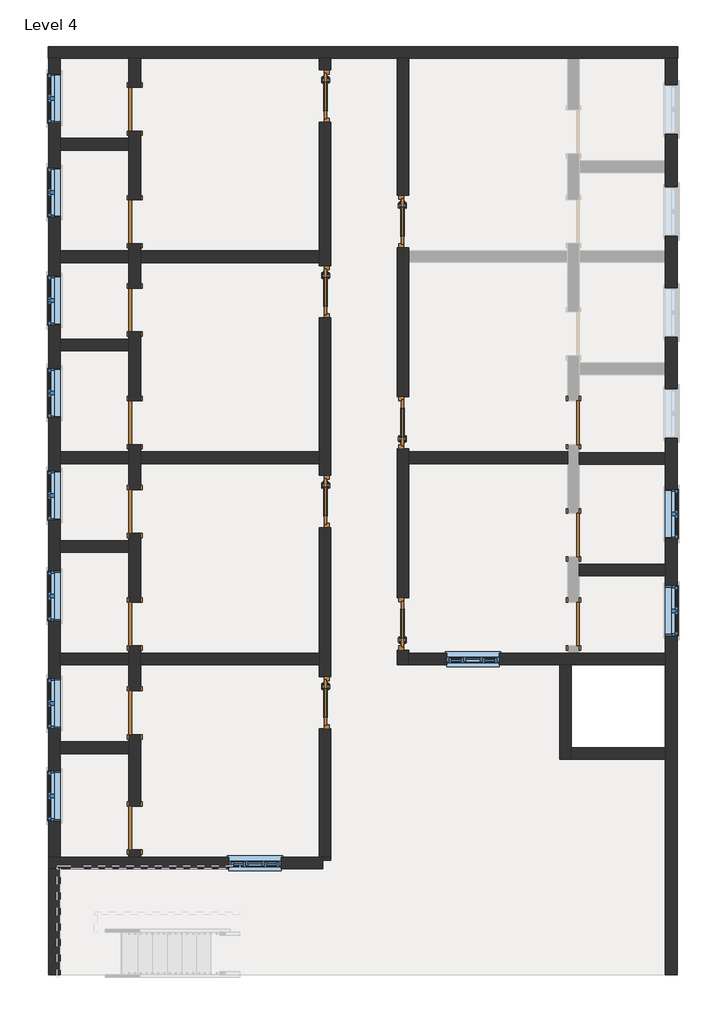
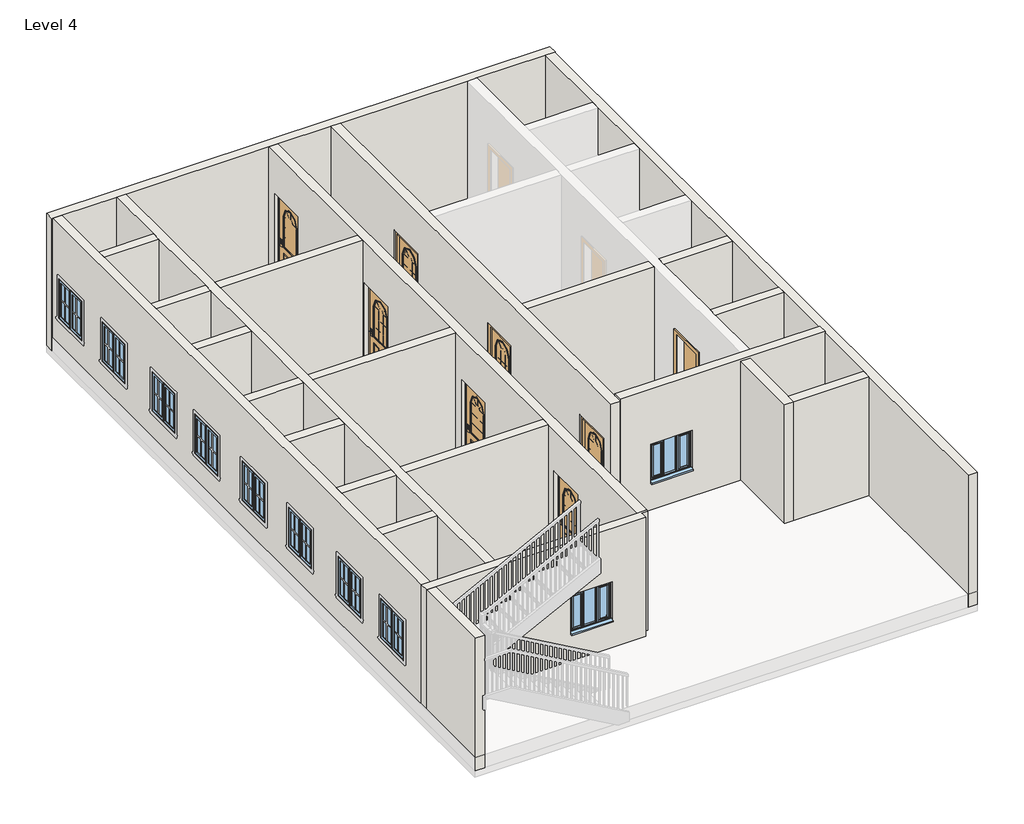
# One storey, part 1 of 4: 24 walls, 18 doors, 12 windows.
"""IFC4 building model written with IfcOpenShell, lengths in millimetres."""

from ifc_helpers import new_model, si_unit, frame, origin, place, context, project, spatial, polyline, outline, extrude, faceted_brep, transform, mapped, element, save
from components import doors_extsgl_w_glazing_bars_arched_910x2110mm_1ab485ba, doors_extsgl_w_glazing_bars_arched_910x2110mm_97dcda8a, door_fadea3f2, door_53b1b562, window_c29befe5, windows_tpl_plain_910x910mm_84e79c20

model = new_model("IFC4")

# Units and contexts
model_context = context("Model", 3, world=origin())
ifc_project = project(units=[si_unit("LENGTHUNIT", "METRE", prefix="MILLI")], contexts=[model_context])

# Site, building, storey
site = spatial("IfcSite", under=ifc_project)
building = spatial("IfcBuilding", under=site)
storey = spatial("IfcBuildingStorey", under=building, Name="Level 4", Elevation=9144.0)

# Doors
placement = place(None, origin())
doors_extsgl_w_glazing_bars_arched_910x2110mm_shape = doors_extsgl_w_glazing_bars_arched_910x2110mm_1ab485ba(model_context)
element("IfcDoor", 1, ObjectType="Doors_ExtSgl_w-Glazing_Bars_Arched : 910x2110mm", at=placement, inside=storey, context=model_context, shape_type="MappedRepresentation", body=[
    mapped(doors_extsgl_w_glazing_bars_arched_910x2110mm_shape, transform((-1635.1108866, 7135.2399728, 9144.0), x_axis=(0.0, -1.0, 0.0), y_axis=(1.0, 0.0, 0.0), z_axis=(0.0, 0.0, 1.0))),
])
element("IfcDoor", 2, ObjectType="Doors_ExtSgl_w-Glazing_Bars_Arched : 910x2110mm", at=placement, inside=storey, context=model_context, shape_type="MappedRepresentation", body=[
    mapped(doors_extsgl_w_glazing_bars_arched_910x2110mm_shape, transform((-1635.1108866, 3727.1935874, 9144.0), x_axis=(0.0, -1.0, 0.0), y_axis=(1.0, 0.0, 0.0), z_axis=(0.0, 0.0, 1.0))),
])
element("IfcDoor", 3, ObjectType="Doors_ExtSgl_w-Glazing_Bars_Arched : 910x2110mm", at=placement, inside=storey, context=model_context, shape_type="MappedRepresentation", body=[
    mapped(doors_extsgl_w_glazing_bars_arched_910x2110mm_shape, transform((-1635.1108866, 74.0399728, 9144.0), x_axis=(0.0, -1.0, 0.0), y_axis=(1.0, 0.0, 0.0), z_axis=(0.0, 0.0, 1.0))),
])
element("IfcDoor", 4, ObjectType="Doors_ExtSgl_w-Glazing_Bars_Arched : 910x2110mm", at=placement, inside=storey, context=model_context, shape_type="MappedRepresentation", body=[
    mapped(doors_extsgl_w_glazing_bars_arched_910x2110mm_shape, transform((-1635.1108866, -3431.1600272, 9144.0), x_axis=(0.0, -1.0, 0.0), y_axis=(1.0, 0.0, 0.0), z_axis=(0.0, 0.0, 1.0))),
])
element("IfcDoor", 5, ObjectType="Doors_ExtSgl_w-Glazing_Bars_Arched : 910x2110mm", at=placement, inside=storey, context=model_context, shape_type="MappedRepresentation", body=[
    mapped(doors_extsgl_w_glazing_bars_arched_910x2110mm_shape, transform((-276.2108866, -2059.5600272, 9144.0), x_axis=(0.0, 1.0, 0.0), y_axis=(-1.0, 0.0, 0.0), z_axis=(0.0, 0.0, 1.0))),
])
element("IfcDoor", 6, ObjectType="Doors_ExtSgl_w-Glazing_Bars_Arched : 910x2110mm", at=placement, inside=storey, context=model_context, shape_type="MappedRepresentation", body=[
    mapped(doors_extsgl_w_glazing_bars_arched_910x2110mm_shape, transform((-276.2108866, 1445.6399728, 9144.0), x_axis=(0.0, 1.0, 0.0), y_axis=(-1.0, 0.0, 0.0), z_axis=(0.0, 0.0, 1.0))),
])
doors_extsgl_w_glazing_bars_arched_910x2110mm_2_shape = doors_extsgl_w_glazing_bars_arched_910x2110mm_97dcda8a(model_context)
element("IfcDoor", 7, ObjectType="Doors_ExtSgl_w-Glazing_Bars_Arched : 910x2110mm", at=placement, inside=storey, context=model_context, shape_type="MappedRepresentation", body=[
    mapped(doors_extsgl_w_glazing_bars_arched_910x2110mm_2_shape, transform((-276.2108866, 4950.8399728, 9144.0), x_axis=(0.0, -1.0, 0.0), y_axis=(1.0, 0.0, 0.0), z_axis=(0.0, 0.0, 1.0))),
])
door_shape = door_fadea3f2(model_context)
element("IfcDoor", 8, ObjectType="Single-Flush : 30\" x 80\"", at=placement, inside=storey, context=model_context, shape_type="MappedRepresentation", body=[
    mapped(door_shape, transform((2695.5891134, -510.1600272, 9144.0), x_axis=(0.0, -1.0, 0.0), y_axis=(1.0, 0.0, 0.0), z_axis=(0.0, 0.0, 1.0))),
])
element("IfcDoor", 9, ObjectType="Single-Flush : 30\" x 80\"", at=placement, inside=storey, context=model_context, shape_type="MappedRepresentation", body=[
    mapped(door_shape, transform((2695.5891134, -2059.5600272, 9144.0), x_axis=(0.0, -1.0, 0.0), y_axis=(1.0, 0.0, 0.0), z_axis=(0.0, 0.0, 1.0))),
])
door_2_shape = door_53b1b562(model_context)
element("IfcDoor", 10, ObjectType="Single-Flush : 30\" x 80\"", at=placement, inside=storey, context=model_context, shape_type="MappedRepresentation", body=[
    mapped(door_2_shape, transform((-4949.8108866, 6906.6399728, 9144.0), x_axis=(0.0, -1.0, 0.0), y_axis=(1.0, 0.0, 0.0), z_axis=(0.0, 0.0, 1.0))),
])
element("IfcDoor", 11, ObjectType="Single-Flush : 30\" x 80\"", at=placement, inside=storey, context=model_context, shape_type="MappedRepresentation", body=[
    mapped(door_2_shape, transform((-4949.8108866, 4946.3935874, 9144.0), x_axis=(0.0, -1.0, 0.0), y_axis=(1.0, 0.0, 0.0), z_axis=(0.0, 0.0, 1.0))),
])
element("IfcDoor", 12, ObjectType="Single-Flush : 30\" x 80\"", at=placement, inside=storey, context=model_context, shape_type="MappedRepresentation", body=[
    mapped(door_2_shape, transform((-4949.8108866, 3407.538843, 9144.0), x_axis=(0.0, -1.0, 0.0), y_axis=(1.0, 0.0, 0.0), z_axis=(0.0, 0.0, 1.0))),
])
element("IfcDoor", 13, ObjectType="Single-Flush : 30\" x 80\"", at=placement, inside=storey, context=model_context, shape_type="MappedRepresentation", body=[
    mapped(door_2_shape, transform((-4949.8108866, 1445.6399728, 9144.0), x_axis=(0.0, -1.0, 0.0), y_axis=(1.0, 0.0, 0.0), z_axis=(0.0, 0.0, 1.0))),
])
element("IfcDoor", 14, ObjectType="Single-Flush : 30\" x 80\"", at=placement, inside=storey, context=model_context, shape_type="MappedRepresentation", body=[
    mapped(door_2_shape, transform((-4949.8108866, -103.7600272, 9144.0), x_axis=(0.0, -1.0, 0.0), y_axis=(1.0, 0.0, 0.0), z_axis=(0.0, 0.0, 1.0))),
])
element("IfcDoor", 15, ObjectType="Single-Flush : 30\" x 80\"", at=placement, inside=storey, context=model_context, shape_type="MappedRepresentation", body=[
    mapped(door_2_shape, transform((-4949.8108866, -2059.5600272, 9144.0), x_axis=(0.0, -1.0, 0.0), y_axis=(1.0, 0.0, 0.0), z_axis=(0.0, 0.0, 1.0))),
])
element("IfcDoor", 16, ObjectType="Single-Flush : 30\" x 80\"", at=placement, inside=storey, context=model_context, shape_type="MappedRepresentation", body=[
    mapped(door_2_shape, transform((-4949.8108866, -3608.9600272, 9144.0), x_axis=(0.0, -1.0, 0.0), y_axis=(1.0, 0.0, 0.0), z_axis=(0.0, 0.0, 1.0))),
])
element("IfcDoor", 17, ObjectType="Single-Flush : 30\" x 80\"", at=placement, inside=storey, context=model_context, shape_type="MappedRepresentation", body=[
    mapped(door_2_shape, transform((-4949.8108866, -5615.5600272, 9144.0), x_axis=(0.0, -1.0, 0.0), y_axis=(1.0, 0.0, 0.0), z_axis=(0.0, 0.0, 1.0))),
])
element("IfcDoor", 18, ObjectType="Single-Flush : 30\" x 80\"", at=placement, inside=storey, context=model_context, shape_type="MappedRepresentation", body=[
    mapped(door_2_shape, transform((2695.5891134, 1445.6399728, 9144.0), x_axis=(0.0, 1.0, 0.0), y_axis=(-1.0, 0.0, 0.0), z_axis=(0.0, 0.0, 1.0))),
])

# Walls
element("IfcWall", 19, ObjectType="4.5\" p", at=placement, inside=storey, context=model_context, shape_type="Brep", body=[
    faceted_brep([(-5051.4108866, -5996.5600272, 11176.0), (-5051.4108866, -5996.5600272, 9144.0), (-5051.4108866, -6123.5600272, 9144.0), (-5051.4108866, -6123.5600272, 12192.0), (-5051.4108866, -4320.1600272, 12192.0), (-5051.4108866, -4116.9600272, 12192.0), (-5051.4108866, -2770.7600272, 12192.0), (-5051.4108866, -2567.5600272, 12192.0), (-5051.4108866, -814.9600272, 12192.0), (-5051.4108866, -611.7600272, 12192.0), (-5051.4108866, 734.4399728, 12192.0), (-5051.4108866, 937.6399728, 12192.0), (-5051.4108866, 2696.338843, 12192.0), (-5051.4108866, 2899.538843, 12192.0), (-5051.4108866, 4235.1935874, 12192.0), (-5051.4108866, 4438.3935874, 12192.0), (-5051.4108866, 6195.4399728, 12192.0), (-5051.4108866, 6398.6399728, 12192.0), (-5051.4108866, 7795.6399728, 12192.0), (-5051.4108866, 7795.6399728, 9144.0), (-5051.4108866, 7287.6399728, 9144.0), (-5051.4108866, 7287.6399728, 11176.0), (-5051.4108866, 6525.6399728, 11176.0), (-5051.4108866, 6525.6399728, 9144.0), (-5051.4108866, 6398.6399728, 9144.0), (-5051.4108866, 6195.4399728, 9144.0), (-5051.4108866, 5327.3935874, 9144.0), (-5051.4108866, 5327.3935874, 11176.0), (-5051.4108866, 4565.3935874, 11176.0), (-5051.4108866, 4565.3935874, 9144.0), (-5051.4108866, 4438.3935874, 9144.0), (-5051.4108866, 4235.1935874, 9144.0), (-5051.4108866, 3788.538843, 9144.0), (-5051.4108866, 3788.538843, 11176.0), (-5051.4108866, 3026.538843, 11176.0), (-5051.4108866, 3026.538843, 9144.0), (-5051.4108866, 2899.538843, 9144.0), (-5051.4108866, 2696.338843, 9144.0), (-5051.4108866, 1826.6399728, 9144.0), (-5051.4108866, 1826.6399728, 11176.0), (-5051.4108866, 1064.6399728, 11176.0), (-5051.4108866, 1064.6399728, 9144.0), (-5051.4108866, 937.6399728, 9144.0), (-5051.4108866, 734.4399728, 9144.0), (-5051.4108866, 277.2399728, 9144.0), (-5051.4108866, 277.2399728, 11176.0), (-5051.4108866, -484.7600272, 11176.0), (-5051.4108866, -484.7600272, 9144.0), (-5051.4108866, -611.7600272, 9144.0), (-5051.4108866, -814.9600272, 9144.0), (-5051.4108866, -1678.5600272, 9144.0), (-5051.4108866, -1678.5600272, 11176.0), (-5051.4108866, -2440.5600272, 11176.0), (-5051.4108866, -2440.5600272, 9144.0), (-5051.4108866, -2567.5600272, 9144.0), (-5051.4108866, -2770.7600272, 9144.0), (-5051.4108866, -3227.9600272, 9144.0), (-5051.4108866, -3227.9600272, 11176.0), (-5051.4108866, -3989.9600272, 11176.0), (-5051.4108866, -3989.9600272, 9144.0), (-5051.4108866, -4116.9600272, 9144.0), (-5051.4108866, -4320.1600272, 9144.0), (-5051.4108866, -5234.5600272, 9144.0), (-5051.4108866, -5234.5600272, 11176.0), (-4848.2108866, -6123.5600272, 9144.0), (-4848.2108866, -5996.5600272, 9144.0), (-4848.2108866, -5996.5600272, 11176.0), (-4848.2108866, -5234.5600272, 11176.0), (-4848.2108866, -5234.5600272, 9144.0), (-4848.2108866, -3989.9600272, 9144.0), (-4848.2108866, -3989.9600272, 11176.0), (-4848.2108866, -3227.9600272, 11176.0), (-4848.2108866, -3227.9600272, 9144.0), (-4848.2108866, -2770.7600272, 9144.0), (-4848.2108866, -2567.5600272, 9144.0), (-4848.2108866, -2440.5600272, 9144.0), (-4848.2108866, -2440.5600272, 11176.0), (-4848.2108866, -1678.5600272, 11176.0), (-4848.2108866, -1678.5600272, 9144.0), (-4848.2108866, -484.7600272, 9144.0), (-4848.2108866, -484.7600272, 11176.0), (-4848.2108866, 277.2399728, 11176.0), (-4848.2108866, 277.2399728, 9144.0), (-4848.2108866, 734.4399728, 9144.0), (-4848.2108866, 937.6399728, 9144.0), (-4848.2108866, 1064.6399728, 9144.0), (-4848.2108866, 1064.6399728, 11176.0), (-4848.2108866, 1826.6399728, 11176.0), (-4848.2108866, 1826.6399728, 9144.0), (-4848.2108866, 3026.538843, 9144.0), (-4848.2108866, 3026.538843, 11176.0), (-4848.2108866, 3788.538843, 11176.0), (-4848.2108866, 3788.538843, 9144.0), (-4848.2108866, 4235.1935874, 9144.0), (-4848.2108866, 4438.3935874, 9144.0), (-4848.2108866, 4565.3935874, 9144.0), (-4848.2108866, 4565.3935874, 11176.0), (-4848.2108866, 5327.3935874, 11176.0), (-4848.2108866, 5327.3935874, 9144.0), (-4848.2108866, 6525.6399728, 9144.0), (-4848.2108866, 6525.6399728, 11176.0), (-4848.2108866, 7287.6399728, 11176.0), (-4848.2108866, 7287.6399728, 9144.0), (-4848.2108866, 7795.6399728, 9144.0), (-4848.2108866, 7795.6399728, 12192.0), (-4848.2108866, 4438.3935874, 12192.0), (-4848.2108866, 4235.1935874, 12192.0), (-4848.2108866, 937.6399728, 12192.0), (-4848.2108866, 734.4399728, 12192.0), (-4848.2108866, -2567.5600272, 12192.0), (-4848.2108866, -2770.7600272, 12192.0), (-4848.2108866, -6123.5600272, 12192.0)], [[[0, 1, 2, 3, 4, 5, 6, 7, 8, 9, 10, 11, 12, 13, 14, 15, 16, 17, 18, 19, 20, 21, 22, 23, 24, 25, 26, 27, 28, 29, 30, 31, 32, 33, 34, 35, 36, 37, 38, 39, 40, 41, 42, 43, 44, 45, 46, 47, 48, 49, 50, 51, 52, 53, 54, 55, 56, 57, 58, 59, 60, 61, 62, 63]], [[64, 65, 66, 67, 68, 69, 70, 71, 72, 73, 74, 75, 76, 77, 78, 79, 80, 81, 82, 83, 84, 85, 86, 87, 88, 89, 90, 91, 92, 93, 94, 95, 96, 97, 98, 99, 100, 101, 102, 103, 104, 105, 106, 107, 108, 109, 110, 111]], [[20, 19, 103, 102]], [[26, 25, 24, 23, 99, 98]], [[32, 31, 30, 29, 95, 94, 93, 92]], [[38, 37, 36, 35, 89, 88]], [[44, 43, 42, 41, 85, 84, 83, 82]], [[50, 49, 48, 47, 79, 78]], [[56, 55, 54, 53, 75, 74, 73, 72]], [[2, 1, 65, 64]], [[62, 61, 60, 59, 69, 68]], [[18, 17, 16, 15, 14, 13, 12, 11, 10, 9, 8, 7, 6, 5, 4, 3, 111, 110, 109, 108, 107, 106, 105, 104]], [[19, 18, 104, 103]], [[3, 2, 64, 111]], [[100, 99, 23, 22]], [[101, 100, 22, 21]], [[102, 101, 21, 20]], [[96, 95, 29, 28]], [[97, 96, 28, 27]], [[98, 97, 27, 26]], [[90, 89, 35, 34]], [[91, 90, 34, 33]], [[92, 91, 33, 32]], [[86, 85, 41, 40]], [[87, 86, 40, 39]], [[88, 87, 39, 38]], [[80, 79, 47, 46]], [[81, 80, 46, 45]], [[82, 81, 45, 44]], [[76, 75, 53, 52]], [[77, 76, 52, 51]], [[78, 77, 51, 50]], [[70, 69, 59, 58]], [[71, 70, 58, 57]], [[72, 71, 57, 56]], [[66, 65, 1, 0]], [[67, 66, 0, 63]], [[68, 67, 63, 62]]]),
])
element("IfcWall", 20, ObjectType="4.5\" p", at=placement, inside=storey, context=model_context, shape_type="SweptSolid", body=[
    extrude(outline(polyline([(-5051.4108866, 6195.4399728), (-6245.2108866, 6195.4399728), (-6245.2108866, 6398.6399728), (-5051.4108866, 6398.6399728), (-5051.4108866, 6195.4399728)])), frame((0.0, 0.0, 9144.0), z_axis=(0.0, 0.0, 1.0), x_axis=(1.0, 0.0, 0.0)), (0.0, 0.0, 1.0), 3048.0),
])
element("IfcWall", 21, ObjectType="4.5\" p", at=placement, inside=storey, context=model_context, shape_type="SweptSolid", body=[
    extrude(outline(polyline([(-5051.4108866, 4235.1935874), (-6245.2108866, 4235.1935874), (-6245.2108866, 4438.3935874), (-5051.4108866, 4438.3935874), (-5051.4108866, 4235.1935874)])), frame((0.0, 0.0, 9144.0), z_axis=(0.0, 0.0, 1.0), x_axis=(1.0, 0.0, 0.0)), (0.0, 0.0, 1.0), 3048.0),
])
element("IfcWall", 22, ObjectType="4.5\" p", at=placement, inside=storey, context=model_context, shape_type="SweptSolid", body=[
    extrude(outline(polyline([(-5051.4108866, 2696.338843), (-6245.2108866, 2696.338843), (-6245.2108866, 2899.538843), (-5051.4108866, 2899.538843), (-5051.4108866, 2696.338843)])), frame((0.0, 0.0, 9144.0), z_axis=(0.0, 0.0, 1.0), x_axis=(1.0, 0.0, 0.0)), (0.0, 0.0, 1.0), 3048.0),
])
element("IfcWall", 23, ObjectType="4.5\" p", at=placement, inside=storey, context=model_context, shape_type="SweptSolid", body=[
    extrude(outline(polyline([(-5051.4108866, 734.4399728), (-6245.2108866, 734.4399728), (-6245.2108866, 937.6399728), (-5051.4108866, 937.6399728), (-5051.4108866, 734.4399728)])), frame((0.0, 0.0, 9144.0), z_axis=(0.0, 0.0, 1.0), x_axis=(1.0, 0.0, 0.0)), (0.0, 0.0, 1.0), 3048.0),
])
element("IfcWall", 24, ObjectType="4.5\" p", at=placement, inside=storey, context=model_context, shape_type="SweptSolid", body=[
    extrude(outline(polyline([(-5051.4108866, -814.9600272), (-6245.2108866, -814.9600272), (-6245.2108866, -611.7600272), (-5051.4108866, -611.7600272), (-5051.4108866, -814.9600272)])), frame((0.0, 0.0, 9144.0), z_axis=(0.0, 0.0, 1.0), x_axis=(1.0, 0.0, 0.0)), (0.0, 0.0, 1.0), 3048.0),
])
element("IfcWall", 25, ObjectType="4.5\" p", at=placement, inside=storey, context=model_context, shape_type="SweptSolid", body=[
    extrude(outline(polyline([(-5051.4108866, -2770.7600272), (-6245.2108866, -2770.7600272), (-6245.2108866, -2567.5600272), (-5051.4108866, -2567.5600272), (-5051.4108866, -2770.7600272)])), frame((0.0, 0.0, 9144.0), z_axis=(0.0, 0.0, 1.0), x_axis=(1.0, 0.0, 0.0)), (0.0, 0.0, 1.0), 3048.0),
])
element("IfcWall", 26, ObjectType="4.5\" p", at=placement, inside=storey, context=model_context, shape_type="SweptSolid", body=[
    extrude(outline(polyline([(-5051.4108866, -4320.1600272), (-6245.2108866, -4320.1600272), (-6245.2108866, -4116.9600272), (-5051.4108866, -4116.9600272), (-5051.4108866, -4320.1600272)])), frame((0.0, 0.0, 9144.0), z_axis=(0.0, 0.0, 1.0), x_axis=(1.0, 0.0, 0.0)), (0.0, 0.0, 1.0), 3048.0),
])
element("IfcWall", 27, ObjectType="4.5\" p", at=placement, inside=storey, context=model_context, shape_type="Brep", body=[
    faceted_brep([(-1736.7108866, -3886.1600272, 11254.0), (-1736.7108866, -3886.1600272, 9144.0), (-1736.7108866, -6123.5600272, 9144.0), (-1736.7108866, -6123.5600272, 12192.0), (-1736.7108866, -2770.7600272, 12192.0), (-1736.7108866, -2567.5600272, 12192.0), (-1736.7108866, 734.4399728, 12192.0), (-1736.7108866, 937.6399728, 12192.0), (-1736.7108866, 4235.1935874, 12192.0), (-1736.7108866, 4438.3935874, 12192.0), (-1736.7108866, 7795.6399728, 12192.0), (-1736.7108866, 7795.6399728, 9144.0), (-1736.7108866, 7590.2399728, 9144.0), (-1736.7108866, 7590.2399728, 11254.0), (-1736.7108866, 6680.2399728, 11254.0), (-1736.7108866, 6680.2399728, 9144.0), (-1736.7108866, 4438.3935874, 9144.0), (-1736.7108866, 4235.1935874, 9144.0), (-1736.7108866, 4182.1935874, 9144.0), (-1736.7108866, 4182.1935874, 11254.0), (-1736.7108866, 3272.1935874, 11254.0), (-1736.7108866, 3272.1935874, 9144.0), (-1736.7108866, 937.6399728, 9144.0), (-1736.7108866, 734.4399728, 9144.0), (-1736.7108866, 529.0399728, 9144.0), (-1736.7108866, 529.0399728, 11254.0), (-1736.7108866, -380.9600272, 11254.0), (-1736.7108866, -380.9600272, 9144.0), (-1736.7108866, -2567.5600272, 9144.0), (-1736.7108866, -2770.7600272, 9144.0), (-1736.7108866, -2976.1600272, 9144.0), (-1736.7108866, -2976.1600272, 11254.0), (-1533.5108866, -6123.5600272, 9144.0), (-1533.5108866, -3886.1600272, 9144.0), (-1533.5108866, -3886.1600272, 11254.0), (-1533.5108866, -2976.1600272, 11254.0), (-1533.5108866, -2976.1600272, 9144.0), (-1533.5108866, -380.9600272, 9144.0), (-1533.5108866, -380.9600272, 11254.0), (-1533.5108866, 529.0399728, 11254.0), (-1533.5108866, 529.0399728, 9144.0), (-1533.5108866, 3272.1935874, 9144.0), (-1533.5108866, 3272.1935874, 11254.0), (-1533.5108866, 4182.1935874, 11254.0), (-1533.5108866, 4182.1935874, 9144.0), (-1533.5108866, 6680.2399728, 9144.0), (-1533.5108866, 6680.2399728, 11254.0), (-1533.5108866, 7590.2399728, 11254.0), (-1533.5108866, 7590.2399728, 9144.0), (-1533.5108866, 7795.6399728, 9144.0), (-1533.5108866, 7795.6399728, 12192.0), (-1533.5108866, -6123.5600272, 12192.0)], [[[0, 1, 2, 3, 4, 5, 6, 7, 8, 9, 10, 11, 12, 13, 14, 15, 16, 17, 18, 19, 20, 21, 22, 23, 24, 25, 26, 27, 28, 29, 30, 31]], [[32, 33, 34, 35, 36, 37, 38, 39, 40, 41, 42, 43, 44, 45, 46, 47, 48, 49, 50, 51]], [[12, 11, 49, 48]], [[18, 17, 16, 15, 45, 44]], [[24, 23, 22, 21, 41, 40]], [[2, 1, 33, 32]], [[30, 29, 28, 27, 37, 36]], [[10, 9, 8, 7, 6, 5, 4, 3, 51, 50]], [[3, 2, 32, 51]], [[11, 10, 50, 49]], [[48, 47, 13, 12]], [[46, 45, 15, 14]], [[47, 46, 14, 13]], [[44, 43, 19, 18]], [[42, 41, 21, 20]], [[43, 42, 20, 19]], [[40, 39, 25, 24]], [[38, 37, 27, 26]], [[39, 38, 26, 25]], [[36, 35, 31, 30]], [[34, 33, 1, 0]], [[35, 34, 0, 31]]]),
])
element("IfcWall", 28, ObjectType="4.5\" p", at=placement, inside=storey, context=model_context, shape_type="SweptSolid", body=[
    extrude(outline(polyline([(-1736.7108866, 4235.1935874), (-4848.2108866, 4235.1935874), (-4848.2108866, 4438.3935874), (-1736.7108866, 4438.3935874), (-1736.7108866, 4235.1935874)])), frame((0.0, 0.0, 9144.0), z_axis=(0.0, 0.0, 1.0), x_axis=(1.0, 0.0, 0.0)), (0.0, 0.0, 1.0), 3048.0),
])
element("IfcWall", 29, ObjectType="4.5\" p", at=placement, inside=storey, context=model_context, shape_type="SweptSolid", body=[
    extrude(outline(polyline([(-1736.7108866, 734.4399728), (-4848.2108866, 734.4399728), (-4848.2108866, 937.6399728), (-1736.7108866, 937.6399728), (-1736.7108866, 734.4399728)])), frame((0.0, 0.0, 9144.0), z_axis=(0.0, 0.0, 1.0), x_axis=(1.0, 0.0, 0.0)), (0.0, 0.0, 1.0), 3048.0),
])
element("IfcWall", 30, ObjectType="4.5\" p", at=placement, inside=storey, context=model_context, shape_type="SweptSolid", body=[
    extrude(outline(polyline([(-1736.7108866, -2770.7600272), (-4848.2108866, -2770.7600272), (-4848.2108866, -2567.5600272), (-1736.7108866, -2567.5600272), (-1736.7108866, -2770.7600272)])), frame((0.0, 0.0, 9144.0), z_axis=(0.0, 0.0, 1.0), x_axis=(1.0, 0.0, 0.0)), (0.0, 0.0, 1.0), 3048.0),
])
element("IfcWall", 31, ObjectType="4.5\" p", at=placement, inside=storey, context=model_context, shape_type="Brep", body=[
    faceted_brep([(-377.8108866, 4495.8399728, 11254.0), (-377.8108866, 4495.8399728, 9144.0), (-377.8108866, 1900.6399728, 9144.0), (-377.8108866, 1900.6399728, 11254.0), (-377.8108866, 990.6399728, 11254.0), (-377.8108866, 990.6399728, 9144.0), (-377.8108866, -1604.5600272, 9144.0), (-377.8108866, -1604.5600272, 11254.0), (-377.8108866, -2514.5600272, 11254.0), (-377.8108866, -2514.5600272, 9144.0), (-377.8108866, -2770.7600272, 9144.0), (-377.8108866, -2770.7600272, 12192.0), (-377.8108866, 7795.6399728, 12192.0), (-377.8108866, 7795.6399728, 9144.0), (-377.8108866, 5405.8399728, 9144.0), (-377.8108866, 5405.8399728, 11254.0), (-174.6108866, 1900.6399728, 9144.0), (-174.6108866, 4239.6399728, 9144.0), (-174.6108866, 4442.8399728, 9144.0), (-174.6108866, 4495.8399728, 9144.0), (-174.6108866, 4495.8399728, 11254.0), (-174.6108866, 5405.8399728, 11254.0), (-174.6108866, 5405.8399728, 9144.0), (-174.6108866, 7795.6399728, 9144.0), (-174.6108866, 7795.6399728, 12192.0), (-174.6108866, 4442.8399728, 12192.0), (-174.6108866, 4239.6399728, 12192.0), (-174.6108866, 937.6399728, 12192.0), (-174.6108866, 734.4399728, 12192.0), (-174.6108866, -2770.7600272, 12192.0), (-174.6108866, -2770.7600272, 9144.0), (-174.6108866, -2567.5600272, 9144.0), (-174.6108866, -2514.5600272, 9144.0), (-174.6108866, -2514.5600272, 11254.0), (-174.6108866, -1604.5600272, 11254.0), (-174.6108866, -1604.5600272, 9144.0), (-174.6108866, 734.4399728, 9144.0), (-174.6108866, 937.6399728, 9144.0), (-174.6108866, 990.6399728, 9144.0), (-174.6108866, 990.6399728, 11254.0), (-174.6108866, 1900.6399728, 11254.0)], [[[0, 1, 2, 3, 4, 5, 6, 7, 8, 9, 10, 11, 12, 13, 14, 15]], [[16, 17, 18, 19, 20, 21, 22, 23, 24, 25, 26, 27, 28, 29, 30, 31, 32, 33, 34, 35, 36, 37, 38, 39, 40]], [[32, 31, 30, 10, 9]], [[38, 37, 36, 35, 6, 5]], [[14, 13, 23, 22]], [[2, 1, 19, 18, 17, 16]], [[12, 11, 29, 28, 27, 26, 25, 24]], [[13, 12, 24, 23]], [[11, 10, 30, 29]], [[9, 8, 33, 32]], [[7, 6, 35, 34]], [[8, 7, 34, 33]], [[5, 4, 39, 38]], [[3, 2, 16, 40]], [[4, 3, 40, 39]], [[22, 21, 15, 14]], [[20, 19, 1, 0]], [[21, 20, 0, 15]]]),
])
element("IfcWall", 32, ObjectType="4.5\" p", at=placement, inside=storey, context=model_context, shape_type="Brep", body=[
    faceted_brep([(-174.6108866, -2770.7600272, 9144.0), (2454.2891134, -2770.7600272, 9144.0), (2657.4891134, -2770.7600272, 9144.0), (4295.7891134, -2770.7600272, 9144.0), (4295.7891134, -2770.7600272, 12232.1226014), (-174.6108866, -2770.7600272, 12232.1226014), (-174.6108866, -2770.7600272, 12192.0), (1397.9891134, -2770.7600272, 10968.4), (1397.9891134, -2770.7600272, 10058.4), (487.9891134, -2770.7600272, 10058.4), (487.9891134, -2770.7600272, 10968.4), (-174.6108866, -2567.5600272, 9144.0), (-174.6108866, -2567.5600272, 12232.1226014), (4295.7891134, -2567.5600272, 12232.1226014), (4295.7891134, -2567.5600272, 9144.0), (2797.1891134, -2567.5600272, 9144.0), (2593.9891134, -2567.5600272, 9144.0), (1397.9891134, -2567.5600272, 10968.4), (487.9891134, -2567.5600272, 10968.4), (487.9891134, -2567.5600272, 10058.4), (1397.9891134, -2567.5600272, 10058.4)], [[[0, 1, 2, 3, 4, 5, 6], [7, 8, 9, 10]], [[11, 12, 13, 14, 15, 16], [17, 18, 19, 20]], [[3, 2, 1, 0, 11, 16, 15, 14]], [[5, 4, 13, 12]], [[0, 6, 5, 12, 11]], [[4, 3, 14, 13]], [[8, 7, 17, 20]], [[9, 8, 20, 19]], [[10, 9, 19, 18]], [[7, 10, 18, 17]]]),
])
element("IfcWall", 33, ObjectType="4.5\" p", at=placement, inside=storey, context=model_context, shape_type="Brep", body=[
    faceted_brep([(2454.2891134, -2770.7600272, 9144.0), (2454.2891134, -4421.7600272, 9144.0), (2454.2891134, -4421.7600272, 12192.0), (2454.2891134, -2770.7600272, 12192.0), (2657.4891134, -2770.7600272, 9144.0), (2657.4891134, -2770.7600272, 12192.0), (2657.4891134, -4218.5600272, 12192.0), (2657.4891134, -4421.7600272, 12192.0), (2657.4891134, -4421.7600272, 9144.0), (2657.4891134, -4218.5600272, 9144.0)], [[[0, 1, 2, 3]], [[4, 5, 6, 7, 8, 9]], [[1, 0, 4, 9, 8]], [[3, 2, 7, 6, 5]], [[0, 3, 5, 4]], [[2, 1, 8, 7]]]),
])
element("IfcWall", 34, ObjectType="4.5\" p", at=placement, inside=storey, context=model_context, shape_type="SweptSolid", body=[
    extrude(outline(polyline([(2657.4891134, -4218.5600272), (4295.7891134, -4218.5600272), (4295.7891134, -4421.7600272), (2657.4891134, -4421.7600272), (2657.4891134, -4218.5600272)])), frame((0.0, 0.0, 9144.0), z_axis=(0.0, 0.0, 1.0), x_axis=(1.0, 0.0, 0.0)), (0.0, 0.0, 1.0), 3048.0),
])
element("IfcWall", 35, ObjectType="4.5\" p", at=placement, inside=storey, context=model_context, shape_type="SweptSolid", body=[
    extrude(outline(polyline([(4295.7891134, 721.7399728), (2797.1891134, 721.7399728), (2797.1891134, 924.9399728), (4295.7891134, 924.9399728), (4295.7891134, 721.7399728)])), frame((0.0, 0.0, 9144.0), z_axis=(0.0, 0.0, 1.0), x_axis=(1.0, 0.0, 0.0)), (0.0, 0.0, 1.0), 3048.0),
])
element("IfcWall", 36, ObjectType="4.5\" p", at=placement, inside=storey, context=model_context, shape_type="SweptSolid", body=[
    extrude(outline(polyline([(4295.7891134, -1221.3600272), (2797.1891134, -1221.3600272), (2797.1891134, -1018.1600272), (4295.7891134, -1018.1600272), (4295.7891134, -1221.3600272)])), frame((0.0, 0.0, 9144.0), z_axis=(0.0, 0.0, 1.0), x_axis=(1.0, 0.0, 0.0)), (0.0, 0.0, 1.0), 3048.0),
])
element("IfcWall", 37, ObjectType="4.5\" p", at=placement, inside=storey, context=model_context, shape_type="SweptSolid", body=[
    extrude(outline(polyline([(2593.9891134, 734.4399728), (-174.6108866, 734.4399728), (-174.6108866, 937.6399728), (2593.9891134, 937.6399728), (2593.9891134, 734.4399728)])), frame((0.0, 0.0, 9144.0), z_axis=(0.0, 0.0, 1.0), x_axis=(1.0, 0.0, 0.0)), (0.0, 0.0, 1.0), 3048.0),
])
element("IfcWall", 38, ObjectType="4.5\" p", at=placement, inside=storey, context=model_context, shape_type="SweptSolid", body=[
    extrude(outline(polyline([(-6448.4108866, -8168.2600272), (-6448.4108866, -6326.7600272), (-6245.2108866, -6326.7600272), (-6245.2108866, -8168.2600272), (-6448.4108866, -8168.2600272)])), frame((0.0, 0.0, 9144.0), z_axis=(0.0, 0.0, 1.0), x_axis=(1.0, 0.0, 0.0)), (0.0, 0.0, 1.0), 3048.0),
])
element("IfcWall", 39, ObjectType="9\" w", at=placement, inside=storey, context=model_context, shape_type="Brep", body=[
    faceted_brep([(-6461.1108866, 7795.6399728, 9144.0), (-6448.4108866, 7795.6399728, 9144.0), (-6245.2108866, 7795.6399728, 9144.0), (-5051.4108866, 7795.6399728, 9144.0), (-4848.2108866, 7795.6399728, 9144.0), (-1736.7108866, 7795.6399728, 9144.0), (-1533.5108866, 7795.6399728, 9144.0), (-377.8108866, 7795.6399728, 9144.0), (-174.6108866, 7795.6399728, 9144.0), (2593.9891134, 7795.6399728, 9144.0), (2797.1891134, 7795.6399728, 9144.0), (4295.7891134, 7795.6399728, 9144.0), (4498.9891134, 7795.6399728, 9144.0), (4511.6891134, 7795.6399728, 9144.0), (4511.6891134, 7795.6399728, 12192.0), (4498.9891134, 7795.6399728, 12192.0), (4295.7891134, 7795.6399728, 12192.0), (2797.1891134, 7795.6399728, 12192.0), (2593.9891134, 7795.6399728, 12192.0), (-174.6108866, 7795.6399728, 12192.0), (-377.8108866, 7795.6399728, 12192.0), (-1533.5108866, 7795.6399728, 12192.0), (-1736.7108866, 7795.6399728, 12192.0), (-4848.2108866, 7795.6399728, 12192.0), (-5051.4108866, 7795.6399728, 12192.0), (-6245.2108866, 7795.6399728, 12192.0), (-6448.4108866, 7795.6399728, 12192.0), (-6461.1108866, 7795.6399728, 12192.0), (-6461.1108866, 7998.8399728, 9144.0), (-6461.1108866, 7998.8399728, 12192.0), (4511.6891134, 7998.8399728, 12192.0), (4511.6891134, 7998.8399728, 9144.0)], [[[0, 1, 2, 3, 4, 5, 6, 7, 8, 9, 10, 11, 12, 13, 14, 15, 16, 17, 18, 19, 20, 21, 22, 23, 24, 25, 26, 27]], [[28, 29, 30, 31]], [[13, 12, 11, 10, 9, 8, 7, 6, 5, 4, 3, 2, 1, 0, 28, 31]], [[14, 13, 31, 30]], [[27, 26, 25, 24, 23, 22, 21, 20, 19, 18, 17, 16, 15, 14, 30, 29]], [[0, 27, 29, 28]]]),
])
element("IfcWall", 40, ObjectType="9\" w", at=placement, inside=storey, context=model_context, shape_type="Brep", body=[
    faceted_brep([(-6448.4108866, -6326.7600272, 12192.0), (-6448.4108866, -6326.7600272, 9144.0), (-6245.2108866, -6326.7600272, 9144.0), (-1673.2108866, -6326.7600272, 9144.0), (-1673.2108866, -6326.7600272, 12192.0), (-6245.2108866, -6326.7600272, 12192.0), (-2399.3108866, -6326.7600272, 10968.4), (-2399.3108866, -6326.7600272, 10058.4), (-3309.3108866, -6326.7600272, 10058.4), (-3309.3108866, -6326.7600272, 10968.4), (-1533.5108866, -6123.5600272, 9144.0), (-1736.7108866, -6123.5600272, 9144.0), (-4848.2108866, -6123.5600272, 9144.0), (-5051.4108866, -6123.5600272, 9144.0), (-6245.2108866, -6123.5600272, 9144.0), (-6448.4108866, -6123.5600272, 9144.0), (-6448.4108866, -6123.5600272, 12192.0), (-6245.2108866, -6123.5600272, 12192.0), (-5051.4108866, -6123.5600272, 12192.0), (-4848.2108866, -6123.5600272, 12192.0), (-1736.7108866, -6123.5600272, 12192.0), (-1533.5108866, -6123.5600272, 12192.0), (-2399.3108866, -6123.5600272, 10058.4), (-2399.3108866, -6123.5600272, 10968.4), (-3309.3108866, -6123.5600272, 10968.4), (-3309.3108866, -6123.5600272, 10058.4), (-1533.5108866, -6174.3600272, 9144.0), (-1673.2108866, -6174.3600272, 9144.0), (-1673.2108866, -6174.3600272, 12192.0), (-1533.5108866, -6174.3600272, 12192.0)], [[[0, 1, 2, 3, 4, 5], [6, 7, 8, 9]], [[10, 11, 12, 13, 14, 15, 16, 17, 18, 19, 20, 21], [22, 23, 24, 25]], [[15, 14, 13, 12, 11, 10, 26, 27, 3, 2, 1]], [[21, 20, 19, 18, 17, 16, 0, 5, 4, 28, 29]], [[1, 0, 16, 15]], [[10, 21, 29, 26]], [[7, 6, 23, 22]], [[8, 7, 22, 25]], [[9, 8, 25, 24]], [[6, 9, 24, 23]], [[28, 27, 26, 29]], [[27, 28, 4, 3]]]),
])
element("IfcWall", 41, ObjectType="9\" w", at=placement, inside=storey, context=model_context, shape_type="Brep", body=[
    faceted_brep([(-6448.4108866, 7795.6399728, 9144.0), (-6448.4108866, -6123.5600272, 9144.0), (-6448.4108866, -6123.5600272, 12192.0), (-6448.4108866, 7795.6399728, 12192.0), (-6448.4108866, 7528.9399728, 10972.8), (-6448.4108866, 6665.3399728, 10972.8), (-6448.4108866, 6665.3399728, 10058.4), (-6448.4108866, 7528.9399728, 10058.4), (-6448.4108866, 5890.6399728, 10972.8), (-6448.4108866, 5027.0399728, 10972.8), (-6448.4108866, 5027.0399728, 10058.4), (-6448.4108866, 5890.6399728, 10058.4), (-6448.4108866, 4006.5935874, 10972.8), (-6448.4108866, 3142.9935874, 10972.8), (-6448.4108866, 3142.9935874, 10058.4), (-6448.4108866, 4006.5935874, 10058.4), (-6448.4108866, 2391.538843, 10972.8), (-6448.4108866, 1527.938843, 10972.8), (-6448.4108866, 1527.938843, 10058.4), (-6448.4108866, 2391.538843, 10058.4), (-6448.4108866, 607.4399728, 10972.8), (-6448.4108866, -256.1600272, 10972.8), (-6448.4108866, -256.1600272, 10058.4), (-6448.4108866, 607.4399728, 10058.4), (-6448.4108866, -1145.1600272, 10972.8), (-6448.4108866, -2008.7600272, 10972.8), (-6448.4108866, -2008.7600272, 10058.4), (-6448.4108866, -1145.1600272, 10058.4), (-6448.4108866, -3012.0600272, 10972.8), (-6448.4108866, -3875.6600272, 10972.8), (-6448.4108866, -3875.6600272, 10058.4), (-6448.4108866, -3012.0600272, 10058.4), (-6448.4108866, -4624.9600272, 10972.8), (-6448.4108866, -5488.5600272, 10972.8), (-6448.4108866, -5488.5600272, 10058.4), (-6448.4108866, -4624.9600272, 10058.4), (-6245.2108866, 7795.6399728, 9144.0), (-6245.2108866, 7795.6399728, 12192.0), (-6245.2108866, 6398.6399728, 12192.0), (-6245.2108866, 6195.4399728, 12192.0), (-6245.2108866, 4438.3935874, 12192.0), (-6245.2108866, 4235.1935874, 12192.0), (-6245.2108866, 2899.538843, 12192.0), (-6245.2108866, 2696.338843, 12192.0), (-6245.2108866, 937.6399728, 12192.0), (-6245.2108866, 734.4399728, 12192.0), (-6245.2108866, -611.7600272, 12192.0), (-6245.2108866, -814.9600272, 12192.0), (-6245.2108866, -2567.5600272, 12192.0), (-6245.2108866, -2770.7600272, 12192.0), (-6245.2108866, -4116.9600272, 12192.0), (-6245.2108866, -4320.1600272, 12192.0), (-6245.2108866, -6123.5600272, 12192.0), (-6245.2108866, -6123.5600272, 9144.0), (-6245.2108866, -4320.1600272, 9144.0), (-6245.2108866, -4116.9600272, 9144.0), (-6245.2108866, -2770.7600272, 9144.0), (-6245.2108866, -2567.5600272, 9144.0), (-6245.2108866, -814.9600272, 9144.0), (-6245.2108866, -611.7600272, 9144.0), (-6245.2108866, 734.4399728, 9144.0), (-6245.2108866, 937.6399728, 9144.0), (-6245.2108866, 2696.338843, 9144.0), (-6245.2108866, 2899.538843, 9144.0), (-6245.2108866, 4235.1935874, 9144.0), (-6245.2108866, 4438.3935874, 9144.0), (-6245.2108866, 6195.4399728, 9144.0), (-6245.2108866, 6398.6399728, 9144.0), (-6245.2108866, 7528.9399728, 10972.8), (-6245.2108866, 7528.9399728, 10058.4), (-6245.2108866, 6665.3399728, 10058.4), (-6245.2108866, 6665.3399728, 10972.8), (-6245.2108866, 5890.6399728, 10972.8), (-6245.2108866, 5890.6399728, 10058.4), (-6245.2108866, 5027.0399728, 10058.4), (-6245.2108866, 5027.0399728, 10972.8), (-6245.2108866, 4006.5935874, 10972.8), (-6245.2108866, 4006.5935874, 10058.4), (-6245.2108866, 3142.9935874, 10058.4), (-6245.2108866, 3142.9935874, 10972.8), (-6245.2108866, 2391.538843, 10972.8), (-6245.2108866, 2391.538843, 10058.4), (-6245.2108866, 1527.938843, 10058.4), (-6245.2108866, 1527.938843, 10972.8), (-6245.2108866, 607.4399728, 10972.8), (-6245.2108866, 607.4399728, 10058.4), (-6245.2108866, -256.1600272, 10058.4), (-6245.2108866, -256.1600272, 10972.8), (-6245.2108866, -1145.1600272, 10972.8), (-6245.2108866, -1145.1600272, 10058.4), (-6245.2108866, -2008.7600272, 10058.4), (-6245.2108866, -2008.7600272, 10972.8), (-6245.2108866, -3012.0600272, 10972.8), (-6245.2108866, -3012.0600272, 10058.4), (-6245.2108866, -3875.6600272, 10058.4), (-6245.2108866, -3875.6600272, 10972.8), (-6245.2108866, -4624.9600272, 10972.8), (-6245.2108866, -4624.9600272, 10058.4), (-6245.2108866, -5488.5600272, 10058.4), (-6245.2108866, -5488.5600272, 10972.8)], [[[0, 1, 2, 3], [4, 5, 6, 7], [8, 9, 10, 11], [12, 13, 14, 15], [16, 17, 18, 19], [20, 21, 22, 23], [24, 25, 26, 27], [28, 29, 30, 31], [32, 33, 34, 35]], [[36, 37, 38, 39, 40, 41, 42, 43, 44, 45, 46, 47, 48, 49, 50, 51, 52, 53, 54, 55, 56, 57, 58, 59, 60, 61, 62, 63, 64, 65, 66, 67], [68, 69, 70, 71], [72, 73, 74, 75], [76, 77, 78, 79], [80, 81, 82, 83], [84, 85, 86, 87], [88, 89, 90, 91], [92, 93, 94, 95], [96, 97, 98, 99]], [[1, 0, 36, 67, 66, 65, 64, 63, 62, 61, 60, 59, 58, 57, 56, 55, 54, 53]], [[3, 2, 52, 51, 50, 49, 48, 47, 46, 45, 44, 43, 42, 41, 40, 39, 38, 37]], [[2, 1, 53, 52]], [[0, 3, 37, 36]], [[69, 68, 4, 7]], [[70, 69, 7, 6]], [[71, 70, 6, 5]], [[68, 71, 5, 4]], [[73, 72, 8, 11]], [[74, 73, 11, 10]], [[75, 74, 10, 9]], [[72, 75, 9, 8]], [[77, 76, 12, 15]], [[78, 77, 15, 14]], [[79, 78, 14, 13]], [[76, 79, 13, 12]], [[81, 80, 16, 19]], [[82, 81, 19, 18]], [[83, 82, 18, 17]], [[80, 83, 17, 16]], [[85, 84, 20, 23]], [[86, 85, 23, 22]], [[87, 86, 22, 21]], [[84, 87, 21, 20]], [[89, 88, 24, 27]], [[90, 89, 27, 26]], [[91, 90, 26, 25]], [[88, 91, 25, 24]], [[93, 92, 28, 31]], [[94, 93, 31, 30]], [[95, 94, 30, 29]], [[92, 95, 29, 28]], [[97, 96, 32, 35]], [[98, 97, 35, 34]], [[99, 98, 34, 33]], [[96, 99, 33, 32]]]),
])
element("IfcWall", 42, ObjectType="9\" w", at=placement, inside=storey, context=model_context, shape_type="Brep", body=[
    faceted_brep([(4295.7891134, 7795.6399728, 9144.0), (4295.7891134, 6004.9399728, 9144.0), (4295.7891134, 5801.7399728, 9144.0), (4295.7891134, 4442.8399728, 9144.0), (4295.7891134, 4239.6399728, 9144.0), (4295.7891134, 2487.0399728, 9144.0), (4295.7891134, 2283.8399728, 9144.0), (4295.7891134, 924.9399728, 9144.0), (4295.7891134, 721.7399728, 9144.0), (4295.7891134, -1018.1600272, 9144.0), (4295.7891134, -1221.3600272, 9144.0), (4295.7891134, -2567.5600272, 9144.0), (4295.7891134, -2770.7600272, 9144.0), (4295.7891134, -4218.5600272, 9144.0), (4295.7891134, -4421.7600272, 9144.0), (4295.7891134, -8168.2600272, 9144.0), (4295.7891134, -8168.2600272, 12192.0), (4295.7891134, -4421.7600272, 12192.0), (4295.7891134, -4218.5600272, 12192.0), (4295.7891134, -1221.3600272, 12192.0), (4295.7891134, -1018.1600272, 12192.0), (4295.7891134, 721.7399728, 12192.0), (4295.7891134, 924.9399728, 12192.0), (4295.7891134, 2283.8399728, 12192.0), (4295.7891134, 2487.0399728, 12192.0), (4295.7891134, 4239.6399728, 12192.0), (4295.7891134, 4442.8399728, 12192.0), (4295.7891134, 5801.7399728, 12192.0), (4295.7891134, 6004.9399728, 12192.0), (4295.7891134, 7795.6399728, 12192.0), (4295.7891134, -2262.7600272, 10972.8), (4295.7891134, -2262.7600272, 10058.4), (4295.7891134, -1399.1600272, 10058.4), (4295.7891134, -1399.1600272, 10972.8), (4295.7891134, -580.0100272, 10972.8), (4295.7891134, -580.0100272, 10058.4), (4295.7891134, 283.5899728, 10058.4), (4295.7891134, 283.5899728, 10972.8), (4295.7891134, 1172.5899728, 10972.8), (4295.7891134, 1172.5899728, 10058.4), (4295.7891134, 2036.1899728, 10058.4), (4295.7891134, 2036.1899728, 10972.8), (4295.7891134, 2931.5399728, 10972.8), (4295.7891134, 2931.5399728, 10058.4), (4295.7891134, 3795.1399728, 10058.4), (4295.7891134, 3795.1399728, 10972.8), (4295.7891134, 4690.4899728, 10972.8), (4295.7891134, 4690.4899728, 10058.4), (4295.7891134, 5554.0899728, 10058.4), (4295.7891134, 5554.0899728, 10972.8), (4295.7891134, 6468.4899728, 10972.8), (4295.7891134, 6468.4899728, 10058.4), (4295.7891134, 7332.0899728, 10058.4), (4295.7891134, 7332.0899728, 10972.8), (4498.9891134, 7795.6399728, 9144.0), (4498.9891134, 7795.6399728, 12192.0), (4498.9891134, -8168.2600272, 12192.0), (4498.9891134, -8168.2600272, 9144.0), (4498.9891134, -2262.7600272, 10972.8), (4498.9891134, -1399.1600272, 10972.8), (4498.9891134, -1399.1600272, 10058.4), (4498.9891134, -2262.7600272, 10058.4), (4498.9891134, -580.0100272, 10972.8), (4498.9891134, 283.5899728, 10972.8), (4498.9891134, 283.5899728, 10058.4), (4498.9891134, -580.0100272, 10058.4), (4498.9891134, 1172.5899728, 10972.8), (4498.9891134, 2036.1899728, 10972.8), (4498.9891134, 2036.1899728, 10058.4), (4498.9891134, 1172.5899728, 10058.4), (4498.9891134, 2931.5399728, 10972.8), (4498.9891134, 3795.1399728, 10972.8), (4498.9891134, 3795.1399728, 10058.4), (4498.9891134, 2931.5399728, 10058.4), (4498.9891134, 4690.4899728, 10972.8), (4498.9891134, 5554.0899728, 10972.8), (4498.9891134, 5554.0899728, 10058.4), (4498.9891134, 4690.4899728, 10058.4), (4498.9891134, 6468.4899728, 10972.8), (4498.9891134, 7332.0899728, 10972.8), (4498.9891134, 7332.0899728, 10058.4), (4498.9891134, 6468.4899728, 10058.4)], [[[0, 1, 2, 3, 4, 5, 6, 7, 8, 9, 10, 11, 12, 13, 14, 15, 16, 17, 18, 19, 20, 21, 22, 23, 24, 25, 26, 27, 28, 29], [30, 31, 32, 33], [34, 35, 36, 37], [38, 39, 40, 41], [42, 43, 44, 45], [46, 47, 48, 49], [50, 51, 52, 53]], [[54, 55, 56, 57], [58, 59, 60, 61], [62, 63, 64, 65], [66, 67, 68, 69], [70, 71, 72, 73], [74, 75, 76, 77], [78, 79, 80, 81]], [[15, 14, 13, 12, 11, 10, 9, 8, 7, 6, 5, 4, 3, 2, 1, 0, 54, 57]], [[16, 15, 57, 56]], [[29, 28, 27, 26, 25, 24, 23, 22, 21, 20, 19, 18, 17, 16, 56, 55]], [[0, 29, 55, 54]], [[31, 30, 58, 61]], [[32, 31, 61, 60]], [[33, 32, 60, 59]], [[30, 33, 59, 58]], [[35, 34, 62, 65]], [[36, 35, 65, 64]], [[37, 36, 64, 63]], [[34, 37, 63, 62]], [[39, 38, 66, 69]], [[40, 39, 69, 68]], [[41, 40, 68, 67]], [[38, 41, 67, 66]], [[43, 42, 70, 73]], [[44, 43, 73, 72]], [[45, 44, 72, 71]], [[42, 45, 71, 70]], [[47, 46, 74, 77]], [[48, 47, 77, 76]], [[49, 48, 76, 75]], [[46, 49, 75, 74]], [[51, 50, 78, 81]], [[52, 51, 81, 80]], [[53, 52, 80, 79]], [[50, 53, 79, 78]]]),
])

# Windows
window_shape = window_c29befe5(model_context)
element("IfcWindow", 43, ObjectType="Window-Casement-Double : 34\" x 36\"", at=placement, inside=storey, context=model_context, shape_type="MappedRepresentation", body=[
    mapped(window_shape, transform((-6346.8108866, 7097.1399728, 9144.0), x_axis=(0.0, 1.0, 0.0), y_axis=(-1.0, 0.0, 0.0), z_axis=(0.0, 0.0, 1.0))),
])
element("IfcWindow", 44, ObjectType="Window-Casement-Double : 34\" x 36\"", at=placement, inside=storey, context=model_context, shape_type="MappedRepresentation", body=[
    mapped(window_shape, transform((-6346.8108866, 5458.8399728, 9144.0), x_axis=(0.0, 1.0, 0.0), y_axis=(-1.0, 0.0, 0.0), z_axis=(0.0, 0.0, 1.0))),
])
element("IfcWindow", 45, ObjectType="Window-Casement-Double : 34\" x 36\"", at=placement, inside=storey, context=model_context, shape_type="MappedRepresentation", body=[
    mapped(window_shape, transform((-6346.8108866, 3574.7935874, 9144.0), x_axis=(0.0, 1.0, 0.0), y_axis=(-1.0, 0.0, 0.0), z_axis=(0.0, 0.0, 1.0))),
])
element("IfcWindow", 46, ObjectType="Window-Casement-Double : 34\" x 36\"", at=placement, inside=storey, context=model_context, shape_type="MappedRepresentation", body=[
    mapped(window_shape, transform((-6346.8108866, 1959.738843, 9144.0), x_axis=(0.0, 1.0, 0.0), y_axis=(-1.0, 0.0, 0.0), z_axis=(0.0, 0.0, 1.0))),
])
element("IfcWindow", 47, ObjectType="Window-Casement-Double : 34\" x 36\"", at=placement, inside=storey, context=model_context, shape_type="MappedRepresentation", body=[
    mapped(window_shape, transform((-6346.8108866, 175.6399728, 9144.0), x_axis=(0.0, 1.0, 0.0), y_axis=(-1.0, 0.0, 0.0), z_axis=(0.0, 0.0, 1.0))),
])
element("IfcWindow", 48, ObjectType="Window-Casement-Double : 34\" x 36\"", at=placement, inside=storey, context=model_context, shape_type="MappedRepresentation", body=[
    mapped(window_shape, transform((-6346.8108866, -1576.9600272, 9144.0), x_axis=(0.0, 1.0, 0.0), y_axis=(-1.0, 0.0, 0.0), z_axis=(0.0, 0.0, 1.0))),
])
element("IfcWindow", 49, ObjectType="Window-Casement-Double : 34\" x 36\"", at=placement, inside=storey, context=model_context, shape_type="MappedRepresentation", body=[
    mapped(window_shape, transform((-6346.8108866, -3443.8600272, 9144.0), x_axis=(0.0, 1.0, 0.0), y_axis=(-1.0, 0.0, 0.0), z_axis=(0.0, 0.0, 1.0))),
])
element("IfcWindow", 50, ObjectType="Window-Casement-Double : 34\" x 36\"", at=placement, inside=storey, context=model_context, shape_type="MappedRepresentation", body=[
    mapped(window_shape, transform((-6346.8108866, -5056.7600272, 9144.0), x_axis=(0.0, 1.0, 0.0), y_axis=(-1.0, 0.0, 0.0), z_axis=(0.0, 0.0, 1.0))),
])
element("IfcWindow", 51, ObjectType="Window-Casement-Double : 34\" x 36\"", at=placement, inside=storey, context=model_context, shape_type="MappedRepresentation", body=[
    mapped(window_shape, transform((4397.3891134, -1830.9600272, 9144.0), x_axis=(0.0, -1.0, 0.0), y_axis=(1.0, 0.0, 0.0), z_axis=(0.0, 0.0, 1.0))),
])
element("IfcWindow", 52, ObjectType="Window-Casement-Double : 34\" x 36\"", at=placement, inside=storey, context=model_context, shape_type="MappedRepresentation", body=[
    mapped(window_shape, transform((4397.3891134, -148.2100272, 9144.0), x_axis=(0.0, -1.0, 0.0), y_axis=(1.0, 0.0, 0.0), z_axis=(0.0, 0.0, 1.0))),
])
windows_tpl_plain_910x910mm_shape = windows_tpl_plain_910x910mm_84e79c20(model_context)
element("IfcWindow", 53, ObjectType="Windows_Tpl_Plain : 910x910mm", at=placement, inside=storey, context=model_context, shape_type="MappedRepresentation", body=[
    mapped(windows_tpl_plain_910x910mm_shape, transform((516.3224468, -2660.7034594, 8858.4), x_axis=(-1.0, 0.0, 0.0), y_axis=(0.0, -1.0, 0.0), z_axis=(0.0, 0.0, 1.0))),
])
element("IfcWindow", 54, ObjectType="Windows_Tpl_Plain : 910x910mm", at=placement, inside=storey, context=model_context, shape_type="MappedRepresentation", body=[
    mapped(windows_tpl_plain_910x910mm_shape, transform((-3280.9775532, -6216.7034594, 8858.4), x_axis=(-1.0, 0.0, 0.0), y_axis=(0.0, -1.0, 0.0), z_axis=(0.0, 0.0, 1.0))),
])

save(model, "model.ifc")

# Revit data of these elements
# Type "Doors_ExtSgl_w-Glazing_Bars_Arched : 910x2110mm"
#   Type Mark = "19"
#   Type Comments = "External Single"
#   Operation = "SingleSwingRight"
#   Construction Type Id = "SGL"
#   Keynote = "L20"
#   Analytic Construction = "Large single-glazed windows"
#   Wrap Layers (Int) from Ext = 0' - 6.98819"
#   Wrap Layers (Ext) from Ext = 0' - 4.03543"
#   Visual Light Transmittance = 0.9
#   Thickness = 0' - 1.73228"
#   Solar Heat Gain Coefficient = 0.86
#   Rough Width = 2' - 11.82677"
#   Rough Height = 6' - 11.07087"
#   O/A Frame Width = 0' - 2.51969"
#   Heat Transfer Coefficient (U) = 0.979472 BTU/(h·ft²·°F)
#   Handle Z Distance = 3' - 5.33858"
#   Glazing Thickness = 0' - 0.94488"
#   FrameWidth = 0' - 1.65354"
#   FrameOffset - External = 0' - 0.98425"
#   FrameDepth = 0' - 3.50394"
#   Door Panel Width = 2' - 7.77165"
#   Door Panel Thickness = 0' - 1.73228"
#   Door Panel Height = 6' - 6.74016"
#   DONT CHANGE - Half Glazed Width = 0' - 9.98031"
#   DONT CHANGE - Glazed Width = 1' - 7.96063"
#   Cill Thickness = 0' - 2.14567"
#   Cill Projection = 0' - 1.1811"
#   Handle X Distance = 0' - 2.95276"
#   Height = 6' - 11.07087"
#   Structural Tolerance = 0' - 0.25591"
#   Tolerance = 0' - 0.11811"
#   Undercut = 0' - 0.15748"
#   Width = 2' - 11.82677"
#   Cill Extension = 0' - 0.98425"
#   Cavity Closer Width = 0' - 1.9685"
#   Cavity Closer Offset from Ext = 0' - 4.03543"
#   Cavity Closer Depth = 0' - 3.34646"
#   Vis - Ironmongery = yes
#   Vis - Glazing Bars = yes
#   Vis - Cavity Closers = yes
#   Define Thermal Properties by = 1
#   Function = 1
#   Material Glass = Door - Glazing
#   Material Glazing Bar = Door - Panel
#   Material Door = Door - Panel
#   Material Frame = Door - Frame/Mullion
#   Material Ironmongery = Door - Handle
#   Wall Closure = (empty or 0)
# Type "Single-Flush : 30\" x 80\""
#   Type Mark = "5"
#   Construction Type Id = "MDOOR"
#   Assembly Code = "C1020"
#   Analytic Construction = "Metal"
#   Thickness = 0' - 2"
#   Heat Transfer Coefficient (U) = 0.651978 BTU/(h·ft²·°F)
#   Height = 6' - 8"
#   Trim Projection Ext = 0' - 1"
#   Trim Projection Int = 0' - 1"
#   Trim Width = 0' - 3"
#   Width = 2' - 6"
#   Define Thermal Properties by = 1
#   Define Thermal Properties by = 1
#   Door Material = Door - Panel
#   Frame Material = Door - Frame
#   Visual Light Transmittance = 0
#   Solar Heat Gain Coefficient = 0
#   Function = (empty or 0)
#   Wall Closure = (empty or 0)
# Type "4.5\" p"
#   Assembly Code = "B2010"
#   Layers, outside or top first: 0' - 8" no material (function 1)
# Type "9\" w"
#   Assembly Code = "B2010"
#   Layers, outside or top first: 0' - 8" no material (function 1)
# Type "Window-Casement-Double : 34\" x 36\""
#   Type Mark = "14"
#   Fire Rating = "0.5h"
#   Assembly Code = "B2020100"
#   Analytic Construction = "Double glazing - domestic"
#   Frame Extension [instance default] = 0' - 0 1/4"
#   Window Inset [instance default] = 0' - 0"
#   Wall Thickness [instance default] = 0' - 6"
#   Interior Wall Closure [instance default] = 0' - 2 1/4"
#   Half Width = 1' - 5"
#   Visual Light Transmittance = 0.81
#   Thermal Resistance (R) = 1.8146 (h·ft²·°F)/BTU
#   Solar Heat Gain Coefficient = 0.76
#   Rough Width = 2' - 10 1/2"
#   Rough Height = 3' - 0 1/2"
#   Height = 3' - 0"
#   Heat Transfer Coefficient (U) = 0.5511 BTU/(h·ft²·°F)
#   Exterior Wall Closure [instance default] = 0' - 1 1/4"
#   Extension Jamb [instance default] = 0' - 2 1/4"
#   Default Sill Height = 3' - 0"
#   Width = 2' - 10"
#   Define Thermal Properties by = 0
#   Muntin Visibility = yes
#   Interior Trim Visibility [instance default] = yes
#   Exterior Trim Visibility [instance default] = yes
#   Extension Jamb Visibility [instance default] = yes
#   Interior Trim Material = Wood - Stained
#   Muntin Pattern = Muntin Pattern_2x2 : Muntin Pattern_2x2
#   Interior Trim = Trim-Window-Interior-Flat : Picture Frame
#   Interior Frame Material = Wood - Stained
#   Glass Panel Material = Glass
#   Exterior Trim Material = Clad - White
#   Exterior Trim = Trim-Window-Exterior-Flat : with Sill
#   Exterior Frame Material = Clad - White
#   Wall Closure = (empty or 0)
# Type "Windows_Tpl_Plain : 910x910mm"
#   Type Mark = "18"
#   Operation = "TriplePanelVertical"
#   Construction Type Id = "GSP4R"
#   Manufacturer = "Revit"
#   Keynote = "L10"
#   Analytic Construction = "1/8 in Pilkington single glazing"
#   Wrap Layers (Ext) from Ext = 0' - 4.03543"
#   Wrap Layers (Int) from Ext = 0' - 6.98819"
#   Window Board Projection = 0' - 0.98425"
#   Window Board Extension = 0' - 0.98425"
#   Visual Light Transmittance = 0.9
#   Solar Heat Gain Coefficient = 0.78
#   Rough Width = 2' - 11.82677"
#   Rough Height = 2' - 11.82677"
#   Height = 2' - 11.82677"
#   Width = 2' - 11.82677"
#   Heat Transfer Coefficient (U) = 0.6496 BTU/(h·ft²·°F)
#   Glazing Thickness = 0' - 0.94488"
#   FrameOffset - External = 0' - 1.9685"
#   Frame Depth = 0' - 2.55906"
#   Default Head Height = 6' - 11.07087"
#   Cill Depth = 0' - 3.44488"
#   Cavity Closer Width = 0' - 1.9685"
#   Cavity Closer Offset from Ext = 0' - 4.03543"
#   Cavity Closer Depth = 0' - 3.34646"
#   Vis - Cavity Closers = yes
#   Define Thermal Properties by = 1
#   Material Trim = Window Frame
#   Material Glass = Glass
#   Material Frame = Window Frame
#   Wall Closure = (empty or 0)
# Elements 1, 2, 3, 4, 5, 6, 7 (IfcDoor, "Doors_ExtSgl_w-Glazing_Bars_Arched : 910x2110mm")
#   Phase Created = New Construction
#   Materials on its faces: "Door - Panel", "Door - Handle", "Door - Frame/Mullion", "Door - Glazing"
# Elements 8, 9, 10, 11, 12, 13, 14, 15, 16, 17, 18 (IfcDoor, "Single-Flush : 30\" x 80\"")
#   Phase Created = New Construction
#   Materials on its faces: "Door - Frame", "Door - Panel"
# Elements 19, 20, 21, 22, 23, 24, 25, 26, 28, 29, 30, 35, 36, 37 (IfcWall, "4.5\" p")
#   Top Offset = 0' - 0"
#   Base Offset = 0' - 0"
#   wall height = 10' - 0"
#   Phase Created = New Construction
#   Base Constraint = Level 4
#   Top Constraint = Level 5
#   Materials on its faces: "Default Wall"
# Element 27 (IfcWall, "4.5\" p")
#   Top Offset = 0' - 0"
#   Base Offset = 0' - 0"
#   wall height = 10' - 0"
#   Phase Created = New Construction
#   Base Constraint = Level 4
#   Top Constraint = Level 5
#   Materials on its faces: "Default Wall", "Brick, Common"
# Element 31 (IfcWall, "4.5\" p")
#   Top Offset = 0' - 0"
#   Base Offset = 0' - 0"
#   wall height = 10' - 0"
#   Phase Created = New Construction
#   Base Constraint = Level 4
#   Top Constraint = Level 5
#   Materials on its faces: "Default Wall", "Brick, Common", "Window Frame"
# Element 32 (IfcWall, "4.5\" p")
#   Top Offset = 0' - 1.57963"
#   Base Offset = 0' - 0"
#   wall height = 10' - 1.57963"
#   Phase Created = New Construction
#   Base Constraint = Level 4
#   Top Constraint = Level 5
#   Materials on its faces: "Default Wall", "Window Frame"
# Elements 33, 34 (IfcWall, "4.5\" p")
#   Top Offset = 0' - 0"
#   Base Offset = 0' - 0"
#   wall height = 10' - 0"
#   Phase Created = New Construction
#   Base Constraint = Level 4
#   Top Constraint = Level 5
#   Materials on its faces: "Default Wall", "Doors - Glazing Bars"
# Element 38 (IfcWall, "4.5\" p")
#   Top Offset = 0' - 0"
#   Base Offset = 0' - 0"
#   wall height = 10' - 0"
#   Phase Created = New Construction
#   Base Constraint = Level 4
#   Top Constraint = Level 5
#   Materials on its faces: "Default Wall", "Wood - Stained"
# Element 39 (IfcWall, "9\" w")
#   Top Offset = 0' - 0"
#   Base Offset = 0' - 0"
#   wall height = 10' - 0"
#   Phase Created = New Construction
#   Base Constraint = Level 4
#   Top Constraint = Level 5
#   Materials on its faces: "Default Wall", "Cherry", "Wood - Stained"
# Element 40 (IfcWall, "9\" w")
#   Top Offset = 0' - 0"
#   Base Offset = 0' - 0"
#   wall height = 10' - 0"
#   Phase Created = New Construction
#   Base Constraint = Level 4
#   Top Constraint = Level 5
#   Materials on its faces: "Default Wall", "Door - Frame/Mullion", "Wood - Stained", "Brick, Common"
# Element 41 (IfcWall, "9\" w")
#   Top Offset = 0' - 0"
#   Base Offset = 0' - 0"
#   wall height = 10' - 0"
#   Phase Created = New Construction
#   Base Constraint = Level 4
#   Top Constraint = Level 5
#   Materials on its faces: "Default Wall", "Wood - Stained"
